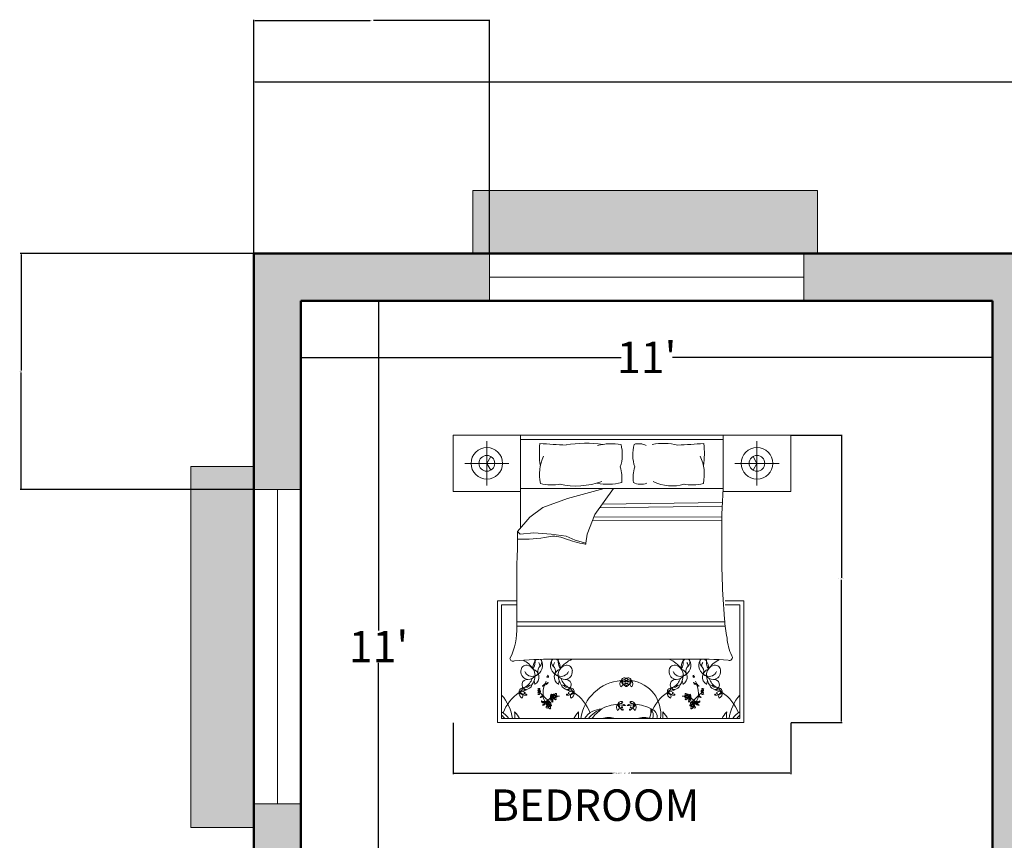
# Model space of a CAD drawing. Units: inches. Extents: x -28 to 544, y -640 to 52.
# Tile 7 of 11: x -28 to 160, y -104 to 52. Entities that reach past the tile are written whole.
import ezdxf

# ---------------------------------------------------------------- set-up
doc = ezdxf.new("R2010")
doc.units = ezdxf.units.IN
doc.header["$MEASUREMENT"] = 0
for name, color, linetype, lineweight in [('A-ANNO-DIMS', 2, 'Continuous', 18), ('A-AREA-IDEN', 7, 'Continuous', 25), ('A-FURN', 8, 'Continuous', 18), ('A-GLAZ', 4, 'Continuous', 20), ('A-ROOF', 8, 'Continuous', 18), ('A-ROOF-PATT', 252, 'Continuous', 13), ('A-WALL', 7, 'Continuous', 50), ('A-WALL-PATT', 5, 'Continuous', 13)]:
    doc.layers.add(name, color=color, linetype=linetype, lineweight=lineweight)
doc.styles.get("Standard").update_dxf_attribs({"font": 'arial.ttf'})
doc.dimstyles.get("Standard").update_dxf_attribs({"dimtxt": 0.18, "dimasz": 0.18, "dimexe": 0.18, "dimexo": 0.0625, "dimgap": 0.09, "dimtad": 0, "dimtih": 1, "dimtoh": 1, "dimdec": 0, "dimzin": 0, "dimdsep": 46, "dimlunit": 3, "dimtxsty": 'Standard', "dimcen": 0.09, "dimadec": 0, "dimazin": 0, "dimtfac": 1, "dimtdec": 0, "dimtofl": 0, "dimtmove": 0, "dimatfit": 3, "dimfxl": 1, "dimtolj": 1, "dimtzin": 0, "dimarcsym": 0})

# ---------------------------------------------------------------- blocks, each defined once
blk = doc.blocks.new('*D1')
at = {"layer": 'A-ANNO-DIMS', "color": 0, "lineweight": -2, "transparency": 16777216}
for p, q in [((40.67, -1.24), (40.56, -1.24)), ((40.74, -1.42), (40.74, -64.14)), ((40.74, -133.06), (40.74, -70.34)), ((40.67, -133.24), (40.56, -133.24))]:
    blk.add_line(p, q, dxfattribs=at)
at = {"layer": 'A-ANNO-DIMS', "color": 0, "transparency": 16777216}
for points in [[(40.71, -1.42), (40.77, -1.42), (40.74, -1.24)], [(40.71, -133.06), (40.77, -133.06), (40.74, -133.24)]]:
    blk.add_solid(points, dxfattribs=at)
at = {"layer": 'Defpoints', "color": 0, "transparency": 16777216}
for p in [(40.74, -1.24), (40.74, -133.24), (40.74, -133.24)]:
    blk.add_point(p, dxfattribs=at)
at = {"layer": 'A-ANNO-DIMS', "color": 0, "transparency": 16777216, "insert": (40.74, -67.24), "char_height": 6, "attachment_point": 5}
blk.add_mtext("\\A1;11'", dxfattribs=at)
blk = doc.blocks.new('*D2')
at = {"layer": 'A-ANNO-DIMS', "color": 0, "lineweight": -2, "transparency": 16777216}
for p, q in [((25.94, -12), (25.94, -11.88)), ((26.12, -12.06), (87.05, -12.06)), ((157.76, -12.06), (96.84, -12.06)), ((157.94, -12), (157.94, -11.88))]:
    blk.add_line(p, q, dxfattribs=at)
at = {"layer": 'A-ANNO-DIMS', "color": 0, "transparency": 16777216}
for points in [[(26.12, -12.03), (26.12, -12.09), (25.94, -12.06)], [(157.76, -12.03), (157.76, -12.09), (157.94, -12.06)]]:
    blk.add_solid(points, dxfattribs=at)
at = {"layer": 'Defpoints', "color": 0, "transparency": 16777216}
for p in [(25.94, -12.06), (157.94, -12.06), (157.94, -12.06)]:
    blk.add_point(p, dxfattribs=at)
at = {"layer": 'A-ANNO-DIMS', "color": 0, "transparency": 16777216, "insert": (91.94, -12.06), "char_height": 6, "attachment_point": 5}
blk.add_mtext("\\A1;11'", dxfattribs=at)
blk = doc.blocks.new('*D27')
at = {"layer": 'A-ANNO-DIMS', "color": 0, "lineweight": -2, "transparency": 16777216}
for p, q in [((16.94, 7.82), (16.94, 40.69)), ((17.12, 40.51), (238.3, 40.51)), ((480.26, 40.51), (259.09, 40.51)), ((480.44, 7.82), (480.44, 40.69))]:
    blk.add_line(p, q, dxfattribs=at)
at = {"layer": 'A-ANNO-DIMS', "color": 0, "transparency": 16777216}
for points in [[(17.12, 40.54), (17.12, 40.48), (16.94, 40.51)], [(480.26, 40.54), (480.26, 40.48), (480.44, 40.51)]]:
    blk.add_solid(points, dxfattribs=at)
at = {"layer": 'Defpoints', "color": 0, "transparency": 16777216}
for p in [(480.44, 40.51), (16.94, 7.76), (480.44, 7.76)]:
    blk.add_point(p, dxfattribs=at)
at = {"layer": 'A-ANNO-DIMS', "color": 0, "transparency": 16777216, "insert": (248.69, 40.51), "char_height": 6, "attachment_point": 5}
blk.add_mtext('\\A1;38\'-8"', dxfattribs=at)
blk = doc.blocks.new('BED-DOUBLE-HEADBOARD-64')
for p, q in [((0, 54.82), (64.46, 54.82)), ((12.89, 54.82), (12.89, 37.12)), ((6.45, 45.23), (6.45, 53.66)), ((51.57, 53.99), (12.89, 53.99)), ((58.01, 45.23), (58.01, 53.66)), ((10.66, 49.44), (2.23, 49.44)), ((53.8, 49.44), (62.22, 49.44)), ((12.89, 44.63), (51.57, 44.63)), ((21.84, 42.71), (28.87, 44.63)), ((30.6, 44.63), (27.07, 39.71)), ((17.14, 41.02), (21.84, 42.71)), ((51.39, 41.95), (28.44, 41.63)), ((14.66, 39.19), (17.14, 41.02)), ((27.07, 39.71), (25.63, 35.93)), ((51.37, 41.29), (27.96, 40.96)), ((12.31, 36.45), (14.66, 39.19)), ((51.34, 38.6), (26.61, 38.5)), ((51.33, 39.26), (26.86, 39.16)), ((12.84, 35.93), (12.31, 36.45)), ((15.45, 36.19), (12.84, 35.93)), ((18.71, 35.93), (15.45, 36.19)), ((21.58, 35.54), (18.71, 35.93)), ((25.63, 35.93), (25.37, 34.23)), ((23.28, 34.76), (21.58, 35.54)), ((25.37, 34.23), (23.28, 34.76)), ((8.51, 23.22), (12.15, 23.22)), ((8.51, 0), (8.51, 23.22)), ((51.92, 23.22), (55.5, 23.22)), ((55.5, 23.22), (55.5, 0)), ((12.15, 22.47), (9.25, 22.47)), ((9.25, 22.47), (9.25, 0.75)), ((54.75, 22.47), (51.91, 22.47)), ((54.75, 0.75), (54.75, 22.47)), ((51.86, 19.2), (12.15, 19.2)), ((51.92, 18.4), (12.15, 18.4)), ((45.31, 12.06), (19.14, 12.06)), ((15.61, 7.28), (15.46, 8.01)), ((20.11, 7.28), (20.25, 8.01)), ((43.9, 7.28), (43.75, 8.01)), ((48.4, 7.28), (48.54, 8.01)), ((55.5, 0), (8.51, 0)), ((9.25, 0.75), (54.75, 0.75))]:
    blk.add_line(p, q)
for points in [[(12.89, 44.07), (0, 44.07), (0, 54.82)], [(51.57, 54.82), (51.57, 44.07), (64.46, 44.07), (64.46, 54.82)], [(6.45, 49.44), (7.2, 50.75)], [(58.01, 49.44), (57.26, 50.75)], [(6.45, 49.44), (7.2, 48.14)], [(58.01, 49.44), (57.26, 48.14)]]:
    blk.add_lwpolyline(points)
for points in [[(16.59, 53.21, 0.074897), (16.67, 49, -0.472817)], [(31.93, 48.76, 0.14099), (32.06, 53.06, 0.235245)], [(34.68, 48.76, -0.14099), (34.55, 53.06, -0.235245)], [(47.86, 53.21, -0.074897), (47.78, 49, 0.472817)], [(12.18, 30.55, 0.001242), (12.15, 18.32, -0.127202), (10.86, 12.22)], [(51.84, 19.71, 0.056112), (52.31, 16.16, 0.095341), (53.21, 12.74)]]:
    blk.add_lwpolyline(points, format="xyb")
for centre, radius in [((6.45, 49.44), 3.01), ((6.45, 49.44), 1.5), ((58.01, 49.44), 3.01), ((58.01, 49.44), 1.5), ((19.33, 4.95), 0.164), ((44.68, 4.95), 0.164), ((18.26, 3.22), 0.164), ((45.75, 3.22), 0.164)]:
    blk.add_circle(centre, radius)
for centre, radius, start, end in [((52.12, 666.62), 614.44, 266.68521, 267.14978), ((25.43, 29.89), 23.38, 82.2196, 99.497), ((30.36, 41.7), 11.49, 81.5249, 103.96), ((35.43, 50), 3.19, 63.3437, 106.1026), ((40.21, 41.93), 11.33, 76.3427, 101.1841), ((12.34, 666.62), 614.44, 272.85022, 273.31479), ((24.81, 47.31), 8.31, 155.1316, 191.7583), ((39.65, 47.31), 8.31, 348.2417, 24.8684), ((24.33, 46.61), 7.9, 354.0129, 15.8293), ((42.28, 46.61), 7.9, 164.1707, 185.9871), ((18.89, 53.96), 8.64, 255.1039, 281.0369), ((23.44, 60.1), 14.98, 258.0397, 289.2615), ((29.51, 56.83), 11.37, 259.8617, 283.6238), ((35.87, 48.88), 3.42, 245.0183, 288.5407), ((41.84, 53.33), 8.2, 243.8761, 286.1746), ((45.56, 53.96), 8.64, 258.9631, 284.8961), ((167.11, 36.75), 115.82, 176.1, 180.9282), ((-46.79, 34.85), 59.12, 355.8294, 1.553), ((13.42, 59.28), 24.33, 267.4519, 281.3392), ((19.23, 30.28), 5.25, 66.2616, 101.3392), ((29.84, 58.59), 25, 250.1194, 259.3383), ((25.22, 34.18), 0.156, 268.8623, 19.7536), ((202.37, 32.54), 151.08, 179.1145, 184.8735), ((11.45, 12.27), 0.595, 183.98, 297.3412), ((18.37, -55.03), 67.1, 89.3433, 95.6887), ((11.2, 7.52), 4.88, 33.6671, 63.2997), ((17.74, 10.43), 2.49, 145.785, 184.7304), ((12.99, 11.59), 2.67, 328.8218, 9.1554), ((16.3, 11.35), 0.776, 120.0293, 142.325), ((15.06, 10.89), 2.05, 289.2822, 29.1751), ((14.75, 10.52), 1.85, 7.436, 29.9149), ((15.97, 11.5), 0.964, 311.5653, 23.8354), ((16.3, 11.35), 0.776, 44.4517, 63.558), ((20.66, 10.89), 2.05, 150.8249, 250.7178), ((19.75, 11.5), 0.964, 156.1646, 228.4347), ((19.42, 11.35), 0.776, 113.229, 135.5483), ((20.97, 10.52), 1.85, 150.0851, 172.564), ((19.42, 11.35), 0.776, 37.675, 66.7144), ((17.98, 10.43), 2.49, 355.2696, 34.215), ((22.73, 11.59), 2.67, 169.7133, 211.1782), ((24.52, 7.52), 4.88, 111.4941, 146.3329), ((39.49, 7.52), 4.88, 33.6671, 68.5059), ((46.03, 10.43), 2.49, 145.785, 184.7304), ((41.28, 11.59), 2.67, 328.8218, 10.2867), ((44.58, 11.35), 0.776, 113.2856, 142.325), ((43.35, 10.89), 2.05, 289.2822, 29.1751), ((43.04, 10.52), 1.85, 7.436, 29.9149), ((44.58, 11.35), 0.776, 44.4517, 66.7144), ((44.26, 11.5), 0.964, 311.5653, 23.8354), ((47.29, -50.63), 62.72, 85.2402, 91.8035), ((48.95, 10.89), 2.05, 150.8249, 250.7178), ((48.04, 11.5), 0.964, 156.1646, 228.4347), ((47.71, 11.35), 0.776, 106.6343, 135.5483), ((49.26, 10.52), 1.85, 150.0851, 172.564), ((47.71, 11.35), 0.776, 37.675, 72.5814), ((46.27, 10.43), 2.49, 355.2696, 34.215), ((51.02, 11.59), 2.67, 169.249, 211.1782), ((52.81, 7.52), 4.88, 113.6453, 146.3329), ((52.73, 12.42), 0.588, 246.5219, 33.8264), ((14.04, 9.87), 1.09, 84.4856, 181.0538), ((14.49, 9.71), 1.54, 174.9449, 262.8857), ((15.09, 10.3), 1.5, 201.5819, 291.4221), ((13.71, 9.06), 1.94, 355.2933, 76.921), ((14.81, 8.67), 1.6, 299.9085, 73.1337), ((15.82, 9.34), 0.4, 257.3041, 15.1471), ((17.48, 9.79), 1.32, 131.5653, 195.1471), ((18.23, 9.79), 1.32, 344.8529, 48.4347), ((20.91, 8.67), 1.6, 106.8663, 240.0915), ((19.9, 9.34), 0.4, 164.8529, 282.6959), ((22.01, 9.06), 1.94, 103.079, 184.7067), ((20.63, 10.3), 1.5, 248.5779, 338.4181), ((21.23, 9.71), 1.54, 277.1143, 5.0551), ((21.68, 9.87), 1.09, 358.9462, 95.5144), ((42.33, 9.87), 1.09, 84.4856, 181.0538), ((42.78, 9.71), 1.54, 174.9449, 262.8857), ((43.38, 10.3), 1.5, 201.5819, 291.4221), ((42, 9.06), 1.94, 355.2933, 76.921), ((43.1, 8.67), 1.6, 299.9085, 73.1337), ((44.11, 9.34), 0.4, 257.3041, 15.1471), ((45.77, 9.79), 1.32, 131.5653, 195.1471), ((46.52, 9.79), 1.32, 344.8529, 48.4347), ((49.2, 8.67), 1.6, 106.8663, 240.0915), ((48.18, 9.34), 0.4, 164.8529, 282.6959), ((50.3, 9.06), 1.94, 103.079, 184.7067), ((48.91, 10.3), 1.5, 248.5779, 338.4181), ((49.52, 9.71), 1.54, 277.1143, 5.0551), ((49.97, 9.87), 1.09, 358.9462, 95.5144), ((14.13, 7.23), 0.967, 80.264, 250.8688), ((12.21, 9.36), 3.04, 301.2614, 341.7045), ((14.22, 10.05), 1.87, 272.3591, 324.0401), ((12.19, 9.11), 3.46, 326.2883, 356.5076), ((17.74, 10.43), 2.49, 212.7011, 216.3445), ((22.51, 5.49), 5.34, 153.0032, 159.8941), ((18.11, 7.28), 0.338, 87.3579, 140.4944), ((17.33, 8.26), 1.02, 301.164, 321.5612), ((18.04, 8.74), 0.124, 102.7051, 280.4384), ((16.5, 8.43), 1.82, 324.6898, 333.4936), ((18.03, 8.81), 0.202, 280.4384, 100.4136), ((17.98, 10.43), 2.49, 323.6555, 327.2989), ((21.5, 10.05), 1.87, 215.9599, 267.6409), ((23.53, 9.11), 3.46, 183.4924, 213.7117), ((23.5, 9.36), 3.04, 198.2955, 238.7386), ((21.59, 7.23), 0.967, 289.1312, 99.736), ((32.73, -0.39), 8.42, 94.4623, 172.255), ((32.77, 7.38), 0.933, 137.7873, 219.1145), ((31.71, 7.41), 0.703, 298.5391, 58.3627), ((32.74, 7.81), 0.698, 63.0274, 163.8037), ((32.04, 9.44), 1.44, 271.4585, 315.3727), ((32.62, 6.79), 1.33, 45.5411, 114.3101), ((33.84, 13.62), 5.89, 252.593, 267.2582), ((32.76, 7.98), 0.689, 177.7585, 283.852), ((34.09, 8.69), 2.13, 198.9159, 238.011), ((33.53, 6.79), 1.33, 65.6899, 134.4589), ((32.32, 13.62), 5.89, 272.7418, 287.407), ((33.41, 7.81), 0.698, 16.1963, 116.9726), ((34.12, 9.44), 1.44, 224.6273, 268.5415), ((32.07, 8.69), 2.13, 301.989, 341.0841), ((33.39, 7.98), 0.689, 256.148, 2.2415), ((34.45, 7.41), 0.703, 121.6373, 241.4609), ((33.39, 7.38), 0.933, 320.8855, 42.2127), ((33.15, 1.56), 6.51, 352.8636, 81.8197), ((42.42, 7.23), 0.967, 80.264, 250.8688), ((40.5, 9.36), 3.04, 301.2614, 341.7045), ((42.51, 10.05), 1.87, 272.3591, 324.0401), ((40.47, 9.11), 3.46, 326.2883, 356.5076), ((46.03, 10.43), 2.49, 212.7011, 216.3445), ((45.98, 8.81), 0.202, 79.5864, 259.5616), ((46.68, 8.26), 1.02, 218.4388, 238.836), ((45.9, 7.28), 0.338, 39.5056, 92.6421), ((47.51, 8.43), 1.82, 206.5064, 215.3102), ((45.96, 8.74), 0.124, 259.5616, 77.2949), ((41.5, 5.49), 5.34, 20.1059, 26.9968), ((46.27, 10.43), 2.49, 323.6555, 327.2989), ((49.79, 10.05), 1.87, 215.9599, 267.6409), ((51.82, 9.11), 3.46, 183.4924, 213.7117), ((51.79, 9.36), 3.04, 198.2955, 238.7386), ((49.87, 7.23), 0.967, 289.1312, 99.736), ((17.39, -1.22), 8.42, 124.3865, 158.5908), ((13.55, 5.53), 0.933, 167.7115, 249.0387), ((13.31, 5.89), 0.698, 92.9516, 193.728), ((11.89, 6.95), 1.44, 301.3827, 345.2969), ((13.71, 4.95), 1.33, 75.4653, 144.2343), ((11.36, 11.48), 5.89, 282.5173, 297.1824), ((12.61, 5.02), 0.703, 328.4633, 88.2869), ((14.04, 7.33), 2.13, 228.8402, 267.9352), ((13.24, 6.05), 0.689, 207.6827, 313.7762), ((13.93, 6.18), 0.593, 63.9755, 143.2681), ((13.66, 5.62), 0.0911, 313.7762, 249.7183), ((13.9, 7.52), 1.21, 265.969, 344.3045), ((15.2, 5.91), 1.29, 96.1662, 141.5825), ((16.38, 6.18), 0.274, 101.5637, 142.6358), ((16.15, 5.92), 0.164, 273.2768, 86.7232), ((16.34, 6.08), 0.157, 91.1081, 181.8675), ((16.66, 5.98), 0.498, 203.4276, 227.6104), ((16.51, 5.76), 0.339, 80.3487, 133.6538), ((16.45, 6.04), 0.269, 229.7889, 317.6792), ((16.16, 6.39), 0.395, 288.7263, 352.5032), ((16.14, 5.47), 0.381, 355.053, 68.3618), ((16.44, 5.41), 0.537, 83.0852, 105.7171), ((16.42, 6.37), 0.127, 345.2356, 144.9248), ((12.72, 0.95), 6.12, 43.1541, 52.0459), ((16.54, 5.96), 0.141, 317.6792, 80.3487), ((17.33, 6.82), 0.338, 101.3256, 154.4621), ((16.85, 7.97), 1.02, 280.2588, 300.656), ((17.08, 8.78), 1.82, 268.3264, 277.1302), ((22.51, 5.49), 5.34, 163.5842, 183.8277), ((16.63, 7.96), 1.04, 308.2101, 316.3071), ((17.26, 7.28), 0.309, 278.3432, 4.2869), ((17.09, 7.55), 0.54, 300.656, 332.6341), ((17.5, 7.2), 0.131, 55.7657, 157.4417), ((17.7, 7.32), 0.131, 84.3784, 186.0543), ((17.58, 7.85), 0.54, 269.1859, 301.164), ((17.74, 7.57), 0.309, 237.5332, 323.4768), ((17.44, 8.45), 1.04, 285.5129, 293.6099), ((20.52, 5.91), 1.29, 38.4175, 83.8338), ((21.82, 7.52), 1.21, 195.6955, 274.031), ((21.78, 6.18), 0.593, 36.7319, 116.0245), ((22, 4.95), 1.33, 35.7657, 104.5347), ((24.36, 11.48), 5.89, 242.8176, 257.4827), ((21.68, 7.33), 2.13, 272.0648, 311.1598), ((22.47, 6.05), 0.689, 226.2238, 332.3173), ((22.07, 5.65), 0.0549, 290.2667, 226.2271), ((23.1, 5.02), 0.703, 91.7131, 211.5367), ((22.41, 5.89), 0.698, 346.272, 87.0484), ((23.83, 6.95), 1.44, 194.7031, 238.6173), ((22.17, 5.53), 0.933, 290.9613, 12.2885), ((18.33, -1.22), 8.42, 21.4092, 55.6135), ((32.91, 7.4), 0.0911, 283.852, 219.9245), ((33.02, 6.98), 0.105, 238.011, 71.5592), ((33.03, 7.03), 0.0508, 71.5592, 188.0167), ((33.14, 6.98), 0.105, 108.4408, 301.989), ((33.12, 7.03), 0.0508, 351.9833, 108.4408), ((33.24, 7.43), 0.0549, 320.1909, 256.0209), ((45.68, -1.22), 8.42, 124.3865, 158.5908), ((41.6, 5.89), 0.698, 92.9516, 193.728), ((41.84, 5.53), 0.933, 167.7115, 249.0387), ((40.18, 6.95), 1.44, 301.3827, 345.2969), ((42, 4.95), 1.33, 75.4653, 144.2343), ((39.65, 11.48), 5.89, 282.5173, 297.1824), ((41.53, 6.05), 0.689, 207.6827, 313.7762), ((42.33, 7.33), 2.13, 228.8402, 267.9352), ((40.9, 5.02), 0.703, 328.4633, 88.2869), ((42.22, 6.18), 0.593, 63.9755, 143.2681), ((41.95, 5.62), 0.0911, 313.7762, 249.7183), ((42.19, 7.52), 1.21, 265.969, 344.3045), ((43.49, 5.91), 1.29, 96.1662, 141.5825), ((46.27, 7.57), 0.309, 216.5232, 302.4668), ((46.43, 7.85), 0.54, 238.836, 270.8141), ((46.57, 8.45), 1.04, 246.3901, 254.4871), ((46.31, 7.32), 0.131, 353.9457, 95.6216), ((46.51, 7.2), 0.131, 22.5583, 124.2343), ((46.75, 7.28), 0.309, 175.7131, 261.6568), ((46.92, 7.55), 0.54, 207.3659, 239.344), ((41.5, 5.49), 5.34, 356.1723, 16.4158), ((47.38, 7.96), 1.04, 223.6929, 231.7899), ((47.16, 7.97), 1.02, 239.344, 259.7412), ((46.93, 8.78), 1.82, 262.8698, 271.6736), ((46.67, 6.82), 0.338, 25.5379, 78.6744), ((51.29, 0.95), 6.12, 127.9541, 136.8459), ((47.47, 5.96), 0.141, 99.6513, 222.3208), ((47.56, 6.04), 0.269, 222.3208, 310.2111), ((47.5, 5.76), 0.339, 46.3462, 99.6513), ((47.58, 6.37), 0.127, 35.0752, 194.7644), ((47.85, 6.39), 0.395, 187.4968, 251.2737), ((47.86, 5.47), 0.381, 111.6382, 184.947), ((47.57, 5.41), 0.537, 74.2829, 96.9148), ((47.67, 6.08), 0.157, 358.1325, 88.8919), ((47.34, 5.98), 0.498, 312.3896, 336.5724), ((47.63, 6.18), 0.274, 37.3642, 78.4363), ((47.86, 5.92), 0.164, 93.2768, 266.7232), ((50.11, 7.52), 1.21, 195.6955, 274.031), ((48.81, 5.91), 1.29, 38.4175, 83.8338), ((50.07, 6.18), 0.593, 36.7319, 116.0245), ((50.29, 4.95), 1.33, 35.7657, 104.5347), ((52.65, 11.48), 5.89, 242.8176, 257.4827), ((49.97, 7.33), 2.13, 272.0648, 311.1598), ((50.76, 6.05), 0.689, 226.2238, 332.3173), ((50.36, 5.65), 0.0549, 290.2667, 226.2271), ((51.39, 5.02), 0.703, 91.7131, 211.5367), ((52.12, 6.95), 1.44, 194.7031, 238.6173), ((50.69, 5.89), 0.698, 346.272, 87.0484), ((50.46, 5.53), 0.933, 290.9613, 12.2885), ((46.62, -1.22), 8.42, 21.4092, 55.6135), ((2.99, -0.39), 8.42, 7.745, 41.8856), ((13.95, 5.36), 0.0508, 101.4834, 217.9409), ((13.96, 5.31), 0.105, 267.9352, 101.4834), ((16.37, 5.62), 0.271, 217.7621, 259.0403), ((16.4, 5.45), 0.126, 232.4737, 355.053), ((16.95, 4.65), 0.338, 101.3256, 154.4621), ((16.46, 5.8), 1.02, 280.2588, 300.656), ((16.7, 6.61), 1.82, 268.3264, 277.1302), ((16.24, 5.79), 1.04, 308.2101, 316.3071), ((17.06, 4.06), 0.183, 146.8636, 236.9021), ((19.65, 8.09), 4.8, 235.1882, 238.8844), ((17.38, 4.32), 0.496, 199.4799, 267.6828), ((16.88, 5.11), 0.309, 278.3432, 4.2869), ((17.32, 4.13), 0.427, 212.8155, 277.3992), ((16.71, 5.39), 0.54, 300.656, 332.6341), ((17.11, 5.03), 0.131, 55.7657, 157.4417), ((17.27, 4.15), 0.19, 238.8844, 314.2646), ((19.85, 5.36), 2.68, 184.756, 209.2041), ((23.71, 11.06), 8.81, 222.2412, 232.1744), ((17.23, 3.72), 0.427, 280.3057, 17.1958), ((17.5, 3.8), 0.143, 19.3605, 201.7548), ((17.5, 3.91), 0.143, 311.8703, 134.2646), ((20.19, 2.61), 2.86, 153.7819, 158.2913), ((17.91, 4.56), 0.748, 247.2305, 319.0635), ((17.67, 4.31), 0.44, 264.4544, 310.6188), ((19.85, 5.36), 2.68, 214.0033, 222.4917), ((17.99, 4.13), 0.455, 218.3208, 298.8162), ((20.13, 1.8), 3.21, 120.544, 139.818), ((18.3, 3.57), 0.529, 70.0041, 130.6188), ((17.96, 4.22), 0.544, 297.7043, 344.3516), ((18.53, 3.67), 0.127, 345.2356, 144.9248), ((18.07, 5.19), 0.748, 304.5369, 16.3699), ((18.47, 5.02), 0.455, 272.8499, 356.1226), ((18.15, 4.85), 0.44, 321.7607, 7.9252), ((18.24, 4.21), 0.44, 8.7227, 54.8872), ((18.27, 3.86), 0.748, 0.278, 72.111), ((19.11, 4.98), 0.529, 127.3105, 187.9252), ((18.6, 4.14), 0.455, 20.5253, 88.5375), ((19.2, 4.36), 0.529, 188.7227, 249.3375), ((18.39, 5.04), 0.544, 355.0106, 41.658), ((18.99, 4.64), 0.163, 148.0499, 225.6268), ((20.13, 1.8), 3.21, 113.0501, 113.8477), ((19.29, 4.45), 0.518, 104.7558, 148.0499), ((19, 4.82), 0.324, 247.4086, 351.4386), ((19.15, 5.17), 0.224, 126.1046, 271.4281), ((19.12, 5.24), 0.161, 353.7526, 131.7054), ((18.52, 4.1), 0.544, 334.9899, 21.6373), ((19.09, 4.81), 0.109, 262.906, 7.132), ((18.97, 5.04), 0.226, 0.0645, 61.1507), ((19.03, 5.24), 0.258, 311.8413, 355.7877), ((19.56, 5.2), 0.274, 101.5637, 176.365), ((19.55, 4.64), 0.271, 151.2196, 259.0403), ((19.52, 5.1), 0.157, 91.1081, 181.8675), ((19.85, 5), 0.498, 203.4276, 227.6104), ((19.69, 4.79), 0.339, 80.3487, 133.6538), ((19.63, 5.07), 0.269, 229.7889, 317.6792), ((19.34, 5.42), 0.395, 288.7263, 352.5032), ((19.32, 4.5), 0.381, 355.053, 68.3618), ((19.62, 4.43), 0.537, 83.0852, 105.7171), ((19.61, 5.4), 0.127, 345.2356, 144.9248), ((19.58, 4.48), 0.126, 232.4737, 355.053), ((19.72, 4.98), 0.141, 317.6792, 80.3487), ((20.13, 1.8), 3.21, 87.1071, 94.7585), ((21.75, 5.31), 0.105, 78.5166, 272.0648), ((21.77, 5.36), 0.0508, 322.0591, 78.5166), ((32.1, 3.3), 0.698, 63.0274, 163.8037), ((31.39, 4.93), 1.44, 271.4585, 315.3727), ((34.06, 3.3), 0.698, 16.1963, 116.9726), ((34.76, 4.93), 1.44, 224.6273, 268.5415), ((42.24, 5.36), 0.0508, 101.4834, 217.9409), ((42.25, 5.31), 0.105, 267.9352, 101.4834), ((43.88, 1.8), 3.21, 85.2415, 92.8929), ((44.29, 4.98), 0.141, 99.6513, 222.3208), ((44.38, 5.07), 0.269, 222.3208, 310.2111), ((44.32, 4.79), 0.339, 46.3462, 99.6513), ((44.4, 5.4), 0.127, 35.0752, 194.7644), ((44.67, 5.42), 0.395, 187.4968, 251.2737), ((44.68, 4.5), 0.381, 111.6382, 184.947), ((44.43, 4.48), 0.126, 184.947, 307.5263), ((44.38, 4.43), 0.537, 74.2829, 96.9148), ((44.49, 5.1), 0.157, 358.1325, 88.8919), ((44.45, 5.2), 0.274, 3.635, 78.4363), ((44.16, 5), 0.498, 312.3896, 336.5724), ((44.45, 4.64), 0.271, 280.9597, 28.7804), ((45.01, 4.82), 0.324, 188.5614, 292.5914), ((44.88, 5.24), 0.161, 48.2946, 186.2474), ((44.98, 5.24), 0.258, 184.2123, 228.1587), ((45.03, 5.04), 0.226, 118.8493, 179.9355), ((44.92, 4.81), 0.109, 172.868, 277.094), ((44.86, 5.17), 0.224, 268.5719, 53.8954), ((44.72, 4.45), 0.518, 31.9501, 75.2442), ((45.48, 4.1), 0.544, 158.3627, 205.0101), ((45.4, 4.14), 0.455, 91.4625, 159.4747), ((45.74, 3.86), 0.748, 107.889, 179.722), ((44.8, 4.36), 0.529, 290.6625, 351.2773), ((45.62, 5.04), 0.544, 138.342, 184.9894), ((45.53, 5.02), 0.455, 183.8774, 267.1501), ((43.88, 1.8), 3.21, 66.1523, 66.9499), ((45.02, 4.64), 0.163, 314.3732, 31.9501), ((45.93, 5.19), 0.748, 163.6301, 235.4631), ((44.89, 4.98), 0.529, 352.0748, 52.6895), ((45.76, 4.21), 0.44, 125.1128, 171.2773), ((45.47, 3.67), 0.127, 35.0752, 194.7644), ((45.85, 4.85), 0.44, 172.0748, 218.2393), ((43.88, 1.8), 3.21, 40.182, 59.456), ((45.71, 3.57), 0.529, 49.3812, 109.9959), ((46.09, 4.56), 0.748, 220.9365, 292.7695), ((46.05, 4.22), 0.544, 195.6484, 242.2957), ((40.3, 11.06), 8.81, 307.8256, 317.7588), ((46.02, 4.13), 0.455, 241.1838, 321.6792), ((46.34, 4.31), 0.44, 229.3812, 275.5456), ((44.15, 5.36), 2.68, 317.5083, 325.9967), ((46.78, 3.72), 0.427, 162.8042, 259.6943), ((46.51, 3.91), 0.143, 45.7354, 228.1297), ((46.51, 3.8), 0.143, 338.2452, 160.6395), ((43.82, 2.61), 2.86, 21.7087, 26.2181), ((44.15, 5.36), 2.68, 330.7959, 355.244), ((46.74, 4.15), 0.19, 225.7354, 301.1156), ((46.69, 4.13), 0.427, 262.6008, 327.1845), ((46.63, 4.32), 0.496, 272.3172, 340.5201), ((46.9, 5.03), 0.131, 22.5583, 124.2343), ((47.13, 5.11), 0.309, 175.7131, 261.6568), ((47.3, 5.39), 0.54, 207.3659, 239.344), ((44.36, 8.09), 4.8, 301.1156, 304.8118), ((47.77, 5.79), 1.04, 223.6929, 231.7899), ((47.55, 5.8), 1.02, 239.344, 259.7412), ((46.94, 4.06), 0.183, 303.0979, 33.1364), ((47.31, 6.61), 1.82, 262.8698, 271.6736), ((47.06, 4.65), 0.338, 25.5379, 78.6744), ((47.61, 5.45), 0.126, 184.947, 307.5263), ((47.64, 5.62), 0.271, 280.9597, 322.2379), ((50.04, 5.31), 0.105, 78.5166, 272.0648), ((50.05, 5.36), 0.0508, 322.0591, 78.5166), ((61.02, -0.39), 8.42, 138.1144, 172.255), ((7.21, -1.51), 4.1, 33.4617, 60.1116), ((9.51, -0.57), 3.42, 22.5547, 48.9546), ((0.13, 1.27), 11.65, 357.4081, 3.6519), ((17.07, 3.85), 0.496, 266.9701, 338.2913), ((14.46, 7.39), 4.8, 302.6784, 306.3746), ((17.2, 3.46), 0.183, 214.3538, 304.3923), ((17.19, 3.68), 0.19, 306.3746, 21.7548), ((17.91, 2.91), 0.163, 148.0499, 225.6268), ((18.21, 2.72), 0.518, 104.7558, 148.0499), ((17.92, 3.09), 0.324, 247.4086, 351.4386), ((18.08, 3.44), 0.224, 126.1046, 271.4281), ((18.05, 3.51), 0.161, 353.7526, 131.7054), ((18.01, 3.08), 0.109, 262.906, 7.132), ((17.9, 3.31), 0.226, 0.0645, 61.1507), ((17.95, 3.51), 0.258, 311.8413, 355.7877), ((18.48, 3.47), 0.274, 101.5637, 176.365), ((18.48, 2.91), 0.271, 151.2196, 259.0403), ((18.45, 3.37), 0.157, 91.1081, 181.8675), ((18.77, 3.27), 0.498, 203.4276, 227.6104), ((18.61, 3.06), 0.339, 80.3487, 133.6538), ((18.55, 3.34), 0.269, 229.7889, 317.6792), ((18.26, 3.68), 0.395, 288.7263, 352.5032), ((18.25, 2.77), 0.381, 355.053, 68.3618), ((18.55, 2.7), 0.537, 83.0852, 105.7171), ((18.51, 2.75), 0.126, 232.4737, 355.053), ((18.65, 3.25), 0.141, 317.6792, 80.3487), ((26.21, -0.57), 3.42, 131.0454, 157.4453), ((35.58, 1.27), 11.65, 176.3481, 182.5919), ((28.51, -1.51), 4.1, 91.272, 146.5383), ((29.98, -2.28), 5.11, 107.8504, 143.6964), ((32.67, -3.72), 7.6, 124.0123, 144.053), ((32.09, -4.9), 8.42, 94.4623, 117.4146), ((32.12, 2.87), 0.933, 137.7873, 219.1145), ((31.06, 2.9), 0.703, 298.5391, 58.3627), ((31.98, 2.28), 1.33, 45.5411, 114.3101), ((33.44, 4.19), 2.13, 198.9159, 238.011), ((33.19, 9.11), 5.89, 252.593, 267.2582), ((32.12, 3.47), 0.689, 177.7585, 283.852), ((32.26, 2.89), 0.0911, 283.852, 219.9245), ((32.37, 2.47), 0.105, 238.011, 71.5592), ((32.39, 2.52), 0.0508, 71.5592, 188.0167), ((34.18, 2.28), 1.33, 65.6899, 134.4589), ((32.96, 9.11), 5.89, 272.7418, 287.407), ((33.78, 2.47), 0.105, 108.4408, 301.989), ((33.77, 2.52), 0.0508, 351.9833, 108.4408), ((33.89, 2.92), 0.0549, 320.1909, 256.0209), ((32.71, 4.19), 2.13, 301.989, 341.0841), ((34.04, 3.47), 0.689, 256.148, 2.2415), ((35.09, 2.9), 0.703, 121.6373, 241.4609), ((34.03, 2.87), 0.933, 320.8855, 42.2127), ((34.07, -4.9), 8.42, 62.5854, 85.5377), ((34, 2.15), 3.77, 338.117, 6.6195), ((37.45, 1.1), 1.51, 346.3898, 79.0739), ((36.32, 1.31), 1.91, 342.8609, 41.9049), ((28.42, 1.27), 11.65, 357.4081, 3.6519), ((37.8, -0.57), 3.42, 22.5547, 48.9546), ((45.36, 3.25), 0.141, 99.6513, 222.3208), ((45.45, 3.34), 0.269, 222.3208, 310.2111), ((45.39, 3.06), 0.339, 46.3462, 99.6513), ((45.74, 3.68), 0.395, 187.4968, 251.2737), ((45.76, 2.77), 0.381, 111.6382, 184.947), ((45.5, 2.75), 0.126, 184.947, 307.5263), ((45.46, 2.7), 0.537, 74.2829, 96.9148), ((45.56, 3.37), 0.157, 358.1325, 88.8919), ((45.23, 3.27), 0.498, 312.3896, 336.5724), ((45.52, 3.47), 0.274, 3.635, 78.4363), ((45.53, 2.91), 0.271, 280.9597, 28.7804), ((46.08, 3.09), 0.324, 188.5614, 292.5914), ((45.96, 3.51), 0.161, 48.2946, 186.2474), ((46.05, 3.51), 0.258, 184.2123, 228.1587), ((46.11, 3.31), 0.226, 118.8493, 179.9355), ((45.99, 3.08), 0.109, 172.868, 277.094), ((45.93, 3.44), 0.224, 268.5719, 53.8954), ((45.79, 2.72), 0.518, 31.9501, 75.2442), ((46.1, 2.91), 0.163, 314.3732, 31.9501), ((46.93, 3.85), 0.496, 201.7087, 273.0299), ((46.82, 3.68), 0.19, 158.2452, 233.6254), ((49.55, 7.39), 4.8, 233.6254, 237.3216), ((46.81, 3.46), 0.183, 235.6077, 325.6462), ((54.5, -0.57), 3.42, 131.0454, 157.4453), ((63.87, 1.27), 11.65, 176.3481, 182.5919), ((56.8, -1.51), 4.1, 119.8884, 146.5383), ((5.74, -2.28), 5.11, 36.3036, 46.4814), ((29.73, -3.68), 4.63, 73.5431, 107.0202), ((31.56, -6.06), 6.84, 94.3787, 95.6357), ((35.17, -10.75), 12.23, 109.7217, 109.9028), ((36.42, -3.68), 4.63, 72.9798, 106.4569), ((34.59, -6.06), 6.84, 84.3643, 85.6213), ((30.99, -10.75), 12.23, 70.0972, 70.2783), ((58.27, -2.28), 5.11, 133.5186, 143.6964)]:
    blk.add_arc(centre, radius, start, end)
blk = doc.blocks.new('WIN-60IN')
for p, q in [((0, 9), (60, 9)), ((0, 0), (0, 9)), ((60, 9), (60, 0)), ((0, 4.5), (60, 4.5)), ((60, 0), (0, 0))]:
    blk.add_line(p, q)
blk = doc.blocks.new('*D65')
at = {"layer": 'A-ANNO-DIMS', "color": 0, "lineweight": -2, "transparency": 16777216}
for p, q in [((54.97, -81.78), (54.97, -91.57)), ((119.42, -81.78), (119.42, -91.57)), ((55.15, -91.39), (85.39, -91.39)), ((119.24, -91.39), (89, -91.39))]:
    blk.add_line(p, q, dxfattribs=at)
at = {"layer": 'A-ANNO-DIMS', "color": 0, "transparency": 16777216}
for points in [[(55.15, -91.36), (55.15, -91.42), (54.97, -91.39)], [(119.24, -91.36), (119.24, -91.42), (119.42, -91.39)]]:
    blk.add_solid(points, dxfattribs=at)
at = {"layer": 'Defpoints', "color": 0, "transparency": 16777216}
for p in [(54.97, -81.72), (119.42, -81.72), (119.42, -91.39)]:
    blk.add_point(p, dxfattribs=at)
at = {"layer": 'A-ANNO-DIMS', "color": 0, "transparency": 16777216, "insert": (87.19, -91.39), "char_height": 0.18, "attachment_point": 5}
blk.add_mtext('\\A1;DOUBLE BED A 5\'-4 1/2" TYP.', dxfattribs=at)
blk = doc.blocks.new('*D66')
at = {"layer": 'A-ANNO-DIMS', "color": 0, "lineweight": -2, "transparency": 16777216}
for p, q in [((119.49, -26.9), (129.27, -26.9)), ((129.09, -27.08), (129.09, -54.13)), ((129.09, -81.54), (129.09, -54.49)), ((119.49, -81.72), (129.27, -81.72))]:
    blk.add_line(p, q, dxfattribs=at)
at = {"layer": 'A-ANNO-DIMS', "color": 0, "transparency": 16777216}
for points in [[(129.06, -27.08), (129.12, -27.08), (129.09, -26.9)], [(129.06, -81.54), (129.12, -81.54), (129.09, -81.72)]]:
    blk.add_solid(points, dxfattribs=at)
at = {"layer": 'Defpoints', "color": 0, "transparency": 16777216}
for p in [(119.42, -26.9), (129.09, -26.9), (119.42, -81.72)]:
    blk.add_point(p, dxfattribs=at)
at = {"layer": 'A-ANNO-DIMS', "color": 0, "transparency": 16777216, "insert": (129.09, -54.31), "char_height": 0.18, "attachment_point": 5}
blk.add_mtext('\\A1;4\'-7" TYP.', dxfattribs=at)
blk = doc.blocks.new('*D86')
at = {"layer": 'A-ANNO-DIMS', "color": 0, "lineweight": -2, "transparency": 16777216}
for p, q in [((16.94, 7.82), (16.94, 52.36)), ((17.12, 52.18), (39.12, 52.18)), ((61.76, 52.18), (39.77, 52.18)), ((61.94, 7.82), (61.94, 52.36))]:
    blk.add_line(p, q, dxfattribs=at)
at = {"layer": 'A-ANNO-DIMS', "color": 0, "transparency": 16777216}
for points in [[(17.12, 52.21), (17.12, 52.15), (16.94, 52.18)], [(61.76, 52.21), (61.76, 52.15), (61.94, 52.18)]]:
    blk.add_solid(points, dxfattribs=at)
at = {"layer": 'Defpoints', "color": 0, "transparency": 16777216}
for p in [(61.94, 52.18), (16.94, 7.76), (61.94, 7.76)]:
    blk.add_point(p, dxfattribs=at)
at = {"layer": 'A-ANNO-DIMS', "color": 0, "transparency": 16777216, "insert": (39.44, 52.18), "char_height": 0.18, "attachment_point": 5}
blk.add_mtext('\\A1;3\'-9"', dxfattribs=at)
blk = doc.blocks.new('*D88')
at = {"layer": 'A-ANNO-DIMS', "color": 0, "lineweight": -2, "transparency": 16777216}
for p, q in [((16.88, 7.76), (-27.66, 7.76)), ((-27.48, 7.58), (-27.48, -14.56)), ((-27.48, -37.06), (-27.48, -14.92)), ((16.88, -37.24), (-27.66, -37.24))]:
    blk.add_line(p, q, dxfattribs=at)
at = {"layer": 'A-ANNO-DIMS', "color": 0, "transparency": 16777216}
for points in [[(-27.51, 7.58), (-27.45, 7.58), (-27.48, 7.76)], [(-27.51, -37.06), (-27.45, -37.06), (-27.48, -37.24)]]:
    blk.add_solid(points, dxfattribs=at)
at = {"layer": 'Defpoints', "color": 0, "transparency": 16777216}
for p in [(16.94, 7.76), (-27.48, -37.24), (16.94, -37.24)]:
    blk.add_point(p, dxfattribs=at)
at = {"layer": 'A-ANNO-DIMS', "color": 0, "transparency": 16777216, "insert": (-27.48, -14.74), "char_height": 0.18, "attachment_point": 5}
blk.add_mtext('\\A1;3\'-9"', dxfattribs=at)

msp = doc.modelspace()

# ---------------------------------------------------------------- hatches: boundary and pattern name
at = {"layer": 'A-ROOF-PATT'}
h = msp.add_hatch(color=256, dxfattribs=at)
h.dxf.hatch_style = 1
h.set_gradient(color1=(241, 235, 31), color2=(248, 153, 30))
h.paths.add_polyline_path([(124.53, 19.76), (58.75, 19.76), (58.75, 7.76), (124.53, 7.76)])
h.paths.add_polyline_path([(226.33, 19.76), (182.83, 19.76), (182.83, 7.76), (226.33, 7.76)])
h.paths.add_polyline_path([(313.67, 19.76), (271.84, 19.76), (271.84, 7.76), (313.67, 7.76)])
h.paths.add_polyline_path([(440.55, 19.76), (372.16, 19.76), (372.16, 7.76), (440.55, 7.76)])
h.paths.add_polyline_path([(492.44, -34.91), (480.44, -34.91), (480.44, -100.18), (492.44, -100.18)])
h.paths.add_polyline_path([(492.44, -151.37), (480.44, -151.37), (480.44, -179.02), (492.44, -179.02)])
h.paths.add_polyline_path([(492.44, -207.96), (480.44, -207.96), (480.44, -238.77), (492.44, -238.77)])
h.paths.add_polyline_path([(492.44, -289.99), (480.44, -289.99), (480.44, -354.53), (492.44, -354.53)])
h.paths.add_polyline_path([(492.44, -399.27), (480.44, -399.27), (480.44, -430), (492.44, -430)])
h.paths.add_polyline_path([(492.44, -475.99), (480.44, -475.99), (480.44, -546.14), (492.44, -546.14)])
h.paths.add_polyline_path([(442.7, -587.74), (368.43, -587.74), (368.43, -599.74), (442.7, -599.74)])
h.paths.add_polyline_path([(127.64, -587.74), (54.75, -587.74), (54.75, -599.74), (127.64, -599.74)])
h.paths.add_polyline_path([(16.94, -477.43), (4.94, -477.43), (4.94, -547.54), (16.94, -547.54)])
h.paths.add_polyline_path([(16.94, -399.8), (4.94, -399.8), (4.94, -430.58), (16.94, -430.58)])
h.paths.add_polyline_path([(16.94, -287.93), (4.94, -287.93), (4.94, -356.82), (16.94, -356.82)])
h.paths.add_polyline_path([(16.94, -208.93), (4.94, -208.93), (4.94, -240.18), (16.94, -240.18)])
h.paths.add_polyline_path([(16.94, -150), (4.94, -150), (4.94, -180.17), (16.94, -180.17)])
h.paths.add_polyline_path([(16.94, -32.89), (4.94, -32.89), (4.94, -101.73), (16.94, -101.73)])
at = {"layer": 'A-WALL-PATT'}
h = msp.add_hatch(color=256, dxfattribs=at)
h.dxf.hatch_style = 1
h.paths.add_polyline_path([(25.94, -235.24), (16.94, -235.24), (16.94, -290.74), (25.94, -290.74), (25.94, -254.74), (127.94, -254.74), (127.94, -252.49), (127.94, -250.24), (118.94, -250.24), (118.94, -247.24), (109.94, -247.24), (109.94, -250.24), (25.94, -250.24)])
h.paths.add_polyline_path([(114.44, -191.74), (114.44, -137.74), (126.94, -137.74), (126.94, -135.49), (126.94, -133.24), (109.94, -133.24), (109.94, -137.74), (109.94, -191.74), (25.94, -191.74), (25.94, -176.74), (16.94, -176.74), (16.94, -211.24), (25.94, -211.24), (25.94, -196.24), (109.94, -196.24), (109.94, -219.24), (114.44, -219.24), (114.44, -196.24)])
h.paths.add_polyline_path([(25.94, -350.74), (16.94, -350.74), (16.94, -403.24), (25.94, -403.24), (25.94, -391.24), (121.94, -391.24), (121.94, -403.24), (126.44, -403.24), (126.44, -391.24), (162.44, -391.24), (162.44, -250.24), (155.94, -250.24), (155.94, -254.74), (157.94, -254.74), (157.94, -386.74), (25.94, -386.74)])
h.paths.add_polyline_path([(25.94, -443.74), (157.94, -443.74), (157.94, -446.74), (162.44, -446.74), (162.44, -439.24), (126.44, -439.24), (126.44, -427.74), (121.94, -427.74), (121.94, -439.24), (25.94, -439.24), (25.94, -427.24), (16.94, -427.24), (16.94, -481.24), (25.94, -481.24)])
h.paths.add_polyline_path([(25.94, -541.24), (16.94, -541.24), (16.94, -587.74), (61.94, -587.74), (61.94, -578.74), (25.94, -578.74)])
h.paths.add_polyline_path([(162.44, -578.74), (162.44, -474.74), (160.19, -474.74), (157.94, -474.74), (157.94, -578.74), (121.94, -578.74), (121.94, -587.74), (162.44, -587.74)])
h.paths.add_polyline_path([(200.69, -578.74), (162.44, -578.74), (162.44, -587.74), (200.69, -587.74)])
h.paths.add_polyline_path([(25.94, -97.24), (16.94, -97.24), (16.94, -152.74), (25.94, -152.74), (25.94, -137.74), (81.94, -137.74), (81.94, -135.49), (81.94, -133.24), (25.94, -133.24)])
h.paths.add_polyline_path([(210.44, -133.24), (162.44, -133.24), (162.44, -1.24), (186.44, -1.24), (186.44, 7.76), (121.94, 7.76), (121.94, -1.24), (157.94, -1.24), (157.94, -133.24), (154.94, -133.24), (154.94, -137.74), (210.44, -137.74)])
h.paths.add_polyline_path([(61.94, 7.76), (16.94, 7.76), (16.94, -37.24), (25.94, -37.24), (25.94, -1.24), (61.94, -1.24)])

# ---------------------------------------------------------------- linework, layer by layer
at = {"layer": 'A-ROOF'}
for p, q in [((58.75, 7.76), (58.75, 19.76)), ((58.75, 19.76), (124.53, 19.76)), ((124.53, 19.76), (124.53, 7.76)), ((4.94, -101.73), (4.94, -32.89)), ((4.94, -32.89), (16.94, -32.89)), ((16.94, -101.73), (4.94, -101.73))]:
    msp.add_line(p, q, dxfattribs=at)
at = {"layer": 'A-WALL'}
for p, q in [((16.94, 7.76), (16.94, -587.74)), ((16.94, 7.76), (480.44, 7.76)), ((25.94, -1.24), (157.94, -1.24)), ((25.94, -1.24), (25.94, -133.24)), ((157.94, -1.24), (157.94, -133.24))]:
    msp.add_line(p, q, dxfattribs=at)

# ---------------------------------------------------------------- block references
at = {"layer": 'A-FURN'}
msp.add_blockref('BED-DOUBLE-HEADBOARD-64', (54.97, -81.72), dxfattribs=at)
at = {"layer": 'A-GLAZ'}
msp.add_blockref('WIN-60IN', (61.95, -1.24), dxfattribs=at)
at = {"layer": 'A-GLAZ', "rotation": 90.00000000000003}
msp.add_blockref('WIN-60IN', (25.94, -97.24), dxfattribs=at)

# ---------------------------------------------------------------- texts
at = {"layer": 'A-AREA-IDEN', "insert": (62.18, -94.49), "char_height": 6, "attachment_point": 1}
msp.add_mtext('BEDROOM', dxfattribs=at)

# ---------------------------------------------------------------- dimensions: what is measured, and where the dimension line sits
at = {"layer": 'A-ANNO-DIMS'}
for base, p1, p2, override, picture, middle in [((61.94, 52.18), (16.94, 7.76), (61.94, 7.76), {"dimdec": 1, "dimlfac": 1, "dimrnd": 0, "dimzin": 1, "dimdsep": 46, "dimlunit": 4, "dimfrac": 2}, '*D86', (39.44, 52.18)), ((480.44473605, 40.50985478), (16.94473605, 7.75882162), (480.44473605, 7.75882162), {"dimtxt": 6, "dimclrd": 0, "dimclre": 0, "dimclrt": 0}, '*D27', (248.69473605, 40.50985478)), ((157.94, -12.06), (25.94, -12.06), (157.94, -12.06), {"dimtxt": 6, "dimclrd": 0, "dimclre": 0, "dimclrt": 0}, '*D2', (91.94, -12.06))]:
    dim = msp.add_linear_dim(base=base, p1=p1, p2=p2, dimstyle='Standard', override=override, dxfattribs=at)
    dim.commit()
    dim.dimension.update_dxf_attribs({"geometry": picture, "text_midpoint": middle})
for base, p1, p2, override, picture, middle in [((-27.48, -37.24), (16.94, 7.76), (16.94, -37.24), {"dimdec": 1, "dimlfac": 1, "dimrnd": 0, "dimzin": 1, "dimdsep": 46, "dimlunit": 4, "dimfrac": 2}, '*D88', (-27.48, -14.74)), ((40.74, -133.24), (40.74, -1.24), (40.74, -133.24), {"dimtxt": 6, "dimclrd": 0, "dimclre": 0, "dimclrt": 0}, '*D1', (40.74, -67.24))]:
    dim = msp.add_linear_dim(base=base, p1=p1, p2=p2, angle=90, dimstyle='Standard', override=override, dxfattribs=at)
    dim.commit()
    dim.dimension.update_dxf_attribs({"geometry": picture, "text_midpoint": middle})
dim = msp.add_linear_dim(base=(129.09, -26.9), p1=(119.42, -81.72), p2=(119.42, -26.9), angle=90, text='<> TYP.', dimstyle='Standard', override={"dimdec": 1, "dimlfac": 1, "dimrnd": 0, "dimzin": 1, "dimdsep": 46, "dimlunit": 4, "dimfrac": 2}, dxfattribs=at)
dim.commit()
dim.dimension.update_dxf_attribs({"geometry": '*D66', "text_midpoint": (129.09, -54.31)})
dim = msp.add_linear_dim(base=(119.4225, -91.388), p1=(54.9663, -81.7196), p2=(119.4225, -81.7196), text='DOUBLE BED A <> TYP.', dimstyle='Standard', override={"dimdec": 1, "dimlfac": 1, "dimrnd": 0, "dimzin": 1, "dimdsep": 46, "dimlunit": 4, "dimfrac": 2}, dxfattribs=at)
dim.commit()
dim.dimension.update_dxf_attribs({"geometry": '*D65', "text_midpoint": (87.1944, -91.388)})

doc.saveas('drawing.dxf')
